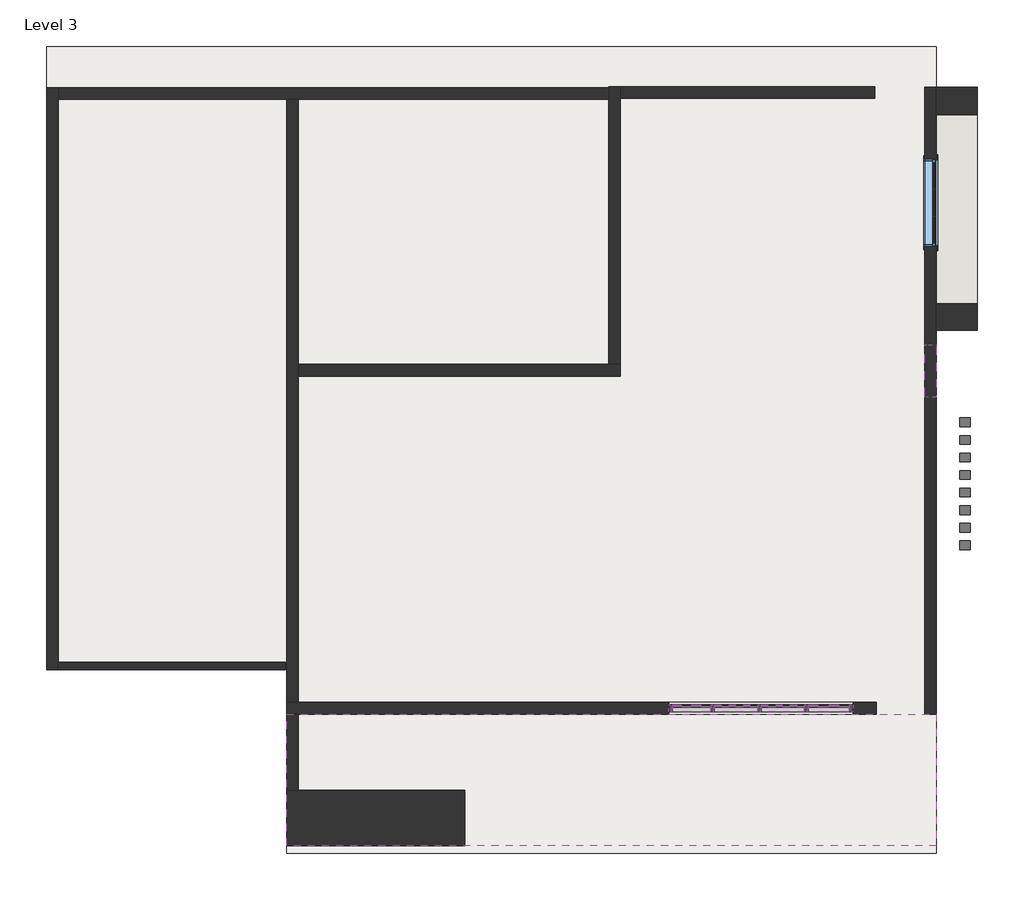
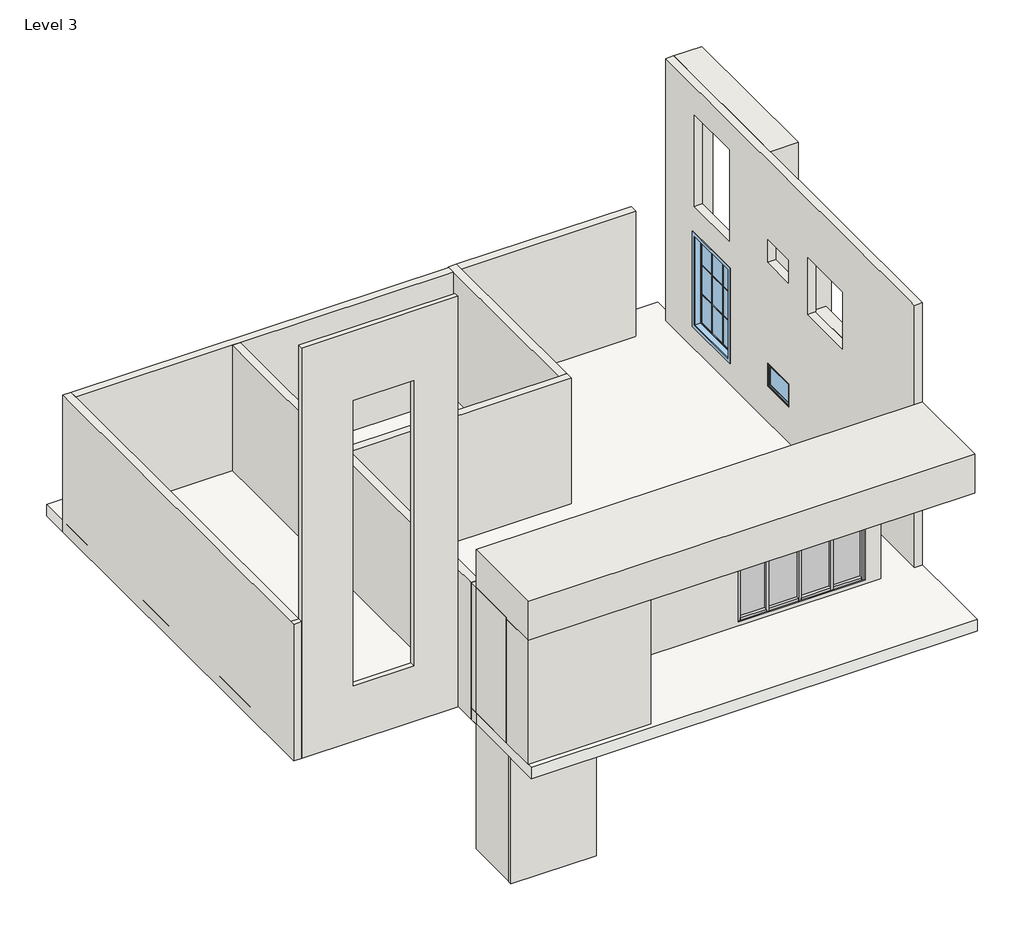
# One storey, incomplete: 22 members, 15 walls, 8 plates, 8 proxies, 2 windows, 1 roof.
"""IFC4 building model written with IfcOpenShell, lengths in millimetres."""

from ifc_helpers import new_model, si_unit, frame, origin, place, context, project, spatial, polyline, outline, extrude, faceted_brep, transform, mapped, element, save
from components import member_424e4c0f, member_61742b2b, member_5ade0aff, member_4d884067, member_c8ba4a72, member_20537117, member_aa870034, member_3a21dca5, member_2ee2964b, member_c33c434a, system_panel_glazed_10e47eeb, system_panel_glazed_d00a1739, system_panel_glazed_0ca22ccd, system_panel_glazed_ae16f783, system_panel_glazed_8c1b86c6, system_panel_glazed_afa25fb8, walls_1_walls_1_5166138d, walls_2_walls_2_a00b9660, walls_3_walls_3_551fdec1, window_41dcc157, window_57c3ee1c

model = new_model("IFC4")

# Units and contexts
model_context = context("Model", 3, world=origin())
ifc_project = project(units=[si_unit("LENGTHUNIT", "METRE", prefix="MILLI")], contexts=[model_context])

# Site, building, storey
site = spatial("IfcSite", under=ifc_project)
building = spatial("IfcBuilding", under=site)
storey = spatial("IfcBuildingStorey", under=building, Name="Level 3", Elevation=7315.2)

# Proxies
placement = place(None, origin())
element("IfcBuildingElementProxy", 1, Name="Reveal", ObjectType="Reveal", at=placement, inside=storey, context=model_context, shape_type="SweptSolid", body=[
    extrude(outline(polyline([(6653.2312442, 1993.3798743), (6470.3512442, 1993.3798743), (6470.3512442, 2145.7798743), (6653.2312442, 2145.7798743), (6653.2312442, 1993.3798743)])), frame((0.0, 0.0, 7620.0), z_axis=(0.0, 0.0, 1.0), x_axis=(1.0, 0.0, 0.0)), (0.0, 0.0, 1.0), 2067.2126797),
])
element("IfcBuildingElementProxy", 2, Name="Reveal", ObjectType="Reveal", at=placement, inside=storey, context=model_context, shape_type="SweptSolid", body=[
    extrude(outline(polyline([(6653.2312442, 2298.1798743), (6470.3512442, 2298.1798743), (6470.3512442, 2450.5798743), (6653.2312442, 2450.5798743), (6653.2312442, 2298.1798743)])), frame((0.0, 0.0, 7620.0), z_axis=(0.0, 0.0, 1.0), x_axis=(1.0, 0.0, 0.0)), (0.0, 0.0, 1.0), 2067.2126797),
])
element("IfcBuildingElementProxy", 3, Name="Reveal", ObjectType="Reveal", at=placement, inside=storey, context=model_context, shape_type="SweptSolid", body=[
    extrude(outline(polyline([(6653.2312442, 2602.9798743), (6470.3512442, 2602.9798743), (6470.3512442, 2755.3798743), (6653.2312442, 2755.3798743), (6653.2312442, 2602.9798743)])), frame((0.0, 0.0, 7620.0), z_axis=(0.0, 0.0, 1.0), x_axis=(1.0, 0.0, 0.0)), (0.0, 0.0, 1.0), 2067.2126797),
])
element("IfcBuildingElementProxy", 4, Name="Reveal", ObjectType="Reveal", at=placement, inside=storey, context=model_context, shape_type="SweptSolid", body=[
    extrude(outline(polyline([(6653.2312442, 2907.7798743), (6470.3512442, 2907.7798743), (6470.3512442, 3060.1798743), (6653.2312442, 3060.1798743), (6653.2312442, 2907.7798743)])), frame((0.0, 0.0, 7620.0), z_axis=(0.0, 0.0, 1.0), x_axis=(1.0, 0.0, 0.0)), (0.0, 0.0, 1.0), 2067.2126797),
])
element("IfcBuildingElementProxy", 5, Name="Reveal", ObjectType="Reveal", at=placement, inside=storey, context=model_context, shape_type="SweptSolid", body=[
    extrude(outline(polyline([(6653.2312442, 3212.5798743), (6470.3512442, 3212.5798743), (6470.3512442, 3364.9798743), (6653.2312442, 3364.9798743), (6653.2312442, 3212.5798743)])), frame((0.0, 0.0, 7620.0), z_axis=(0.0, 0.0, 1.0), x_axis=(1.0, 0.0, 0.0)), (0.0, 0.0, 1.0), 2067.2126797),
])
element("IfcBuildingElementProxy", 6, Name="Reveal", ObjectType="Reveal", at=placement, inside=storey, context=model_context, shape_type="SweptSolid", body=[
    extrude(outline(polyline([(6653.2312442, 3517.3798743), (6470.3512442, 3517.3798743), (6470.3512442, 3669.7798743), (6653.2312442, 3669.7798743), (6653.2312442, 3517.3798743)])), frame((0.0, 0.0, 7620.0), z_axis=(0.0, 0.0, 1.0), x_axis=(1.0, 0.0, 0.0)), (0.0, 0.0, 1.0), 2067.2126797),
])
element("IfcBuildingElementProxy", 7, Name="Reveal", ObjectType="Reveal", at=placement, inside=storey, context=model_context, shape_type="SweptSolid", body=[
    extrude(outline(polyline([(6653.2312442, 3822.1798743), (6470.3512442, 3822.1798743), (6470.3512442, 3974.5798743), (6653.2312442, 3974.5798743), (6653.2312442, 3822.1798743)])), frame((0.0, 0.0, 7620.0), z_axis=(0.0, 0.0, 1.0), x_axis=(1.0, 0.0, 0.0)), (0.0, 0.0, 1.0), 2067.2126797),
])
element("IfcBuildingElementProxy", 8, Name="Reveal", ObjectType="Reveal", at=placement, inside=storey, context=model_context, shape_type="SweptSolid", body=[
    extrude(outline(polyline([(6653.2312442, 4126.9798743), (6470.3512442, 4126.9798743), (6470.3512442, 4279.3798743), (6653.2312442, 4279.3798743), (6653.2312442, 4126.9798743)])), frame((0.0, 0.0, 7620.0), z_axis=(0.0, 0.0, 1.0), x_axis=(1.0, 0.0, 0.0)), (0.0, 0.0, 1.0), 2067.2126797),
])

# Members
member_shape = member_424e4c0f(model_context)
element("IfcMember", 9, ObjectType="Rectangular Mullion : 2.5\" x 5\" rectangular", at=placement, inside=storey, context=model_context, shape_type="MappedRepresentation", body=[
    mapped(member_shape, transform((3771.7551378, -759.3451257, 9949.3840877), x_axis=(0.0, 0.0, 1.0), y_axis=(0.0, -1.0, 0.0), z_axis=(1.0, 0.0, 0.0))),
])
element("IfcMember", 10, ObjectType="Rectangular Mullion : 2.5\" x 5\" rectangular", at=placement, inside=storey, context=model_context, shape_type="MappedRepresentation", body=[
    mapped(member_shape, transform((2958.9382617, -759.3451257, 9949.3840877), x_axis=(0.0, 0.0, 1.0), y_axis=(0.0, -1.0, 0.0), z_axis=(1.0, 0.0, 0.0))),
])
member_2_shape = member_61742b2b(model_context)
element("IfcMember", 11, ObjectType="Rectangular Mullion : 2.5\" x 5\" rectangular", at=placement, inside=storey, context=model_context, shape_type="MappedRepresentation", body=[
    mapped(member_2_shape, transform((2177.8713856, -759.3451257, 9949.3840877), x_axis=(1.0, 0.0, 0.0), y_axis=(0.0, -1.0, 0.0), z_axis=(0.0, 0.0, -1.0))),
])
element("IfcMember", 12, ObjectType="Rectangular Mullion : 2.5\" x 5\" rectangular", at=placement, inside=storey, context=model_context, shape_type="MappedRepresentation", body=[
    mapped(member_2_shape, transform((2990.6882617, -759.3451257, 9949.3840877), x_axis=(1.0, 0.0, 0.0), y_axis=(0.0, -1.0, 0.0), z_axis=(0.0, 0.0, -1.0))),
])
element("IfcMember", 13, ObjectType="Rectangular Mullion : 2.5\" x 5\" rectangular", at=placement, inside=storey, context=model_context, shape_type="MappedRepresentation", body=[
    mapped(member_2_shape, transform((3803.5051378, -759.3451257, 9949.3840877), x_axis=(1.0, 0.0, 0.0), y_axis=(0.0, -1.0, 0.0), z_axis=(0.0, 0.0, -1.0))),
])
member_3_shape = member_5ade0aff(model_context)
element("IfcMember", 14, ObjectType="Rectangular Mullion : 2.5\" x 5\" rectangular", at=placement, inside=storey, context=model_context, shape_type="MappedRepresentation", body=[
    mapped(member_3_shape, transform((3771.7551378, -759.3451257, 10711.3840877), x_axis=(0.0, 0.0, 1.0), y_axis=(0.0, -1.0, 0.0), z_axis=(1.0, 0.0, 0.0))),
])
element("IfcMember", 15, ObjectType="Rectangular Mullion : 2.5\" x 5\" rectangular", at=placement, inside=storey, context=model_context, shape_type="MappedRepresentation", body=[
    mapped(member_3_shape, transform((2958.9382617, -759.3451257, 10711.3840877), x_axis=(0.0, 0.0, 1.0), y_axis=(0.0, -1.0, 0.0), z_axis=(1.0, 0.0, 0.0))),
])
member_4_shape = member_4d884067(model_context)
element("IfcMember", 16, ObjectType="Rectangular Mullion : 2.5\" x 5\" rectangular", at=placement, inside=storey, context=model_context, shape_type="MappedRepresentation", body=[
    mapped(member_4_shape, transform((2177.8713856, -759.3451257, 7721.6), x_axis=(1.0, 0.0, 0.0), y_axis=(0.0, -1.0, 0.0), z_axis=(0.0, 0.0, -1.0))),
])
element("IfcMember", 17, ObjectType="Rectangular Mullion : 2.5\" x 5\" rectangular", at=placement, inside=storey, context=model_context, shape_type="MappedRepresentation", body=[
    mapped(member_4_shape, transform((2990.6882617, -759.3451257, 7721.6), x_axis=(1.0, 0.0, 0.0), y_axis=(0.0, -1.0, 0.0), z_axis=(0.0, 0.0, -1.0))),
])
element("IfcMember", 18, ObjectType="Rectangular Mullion : 2.5\" x 5\" rectangular", at=placement, inside=storey, context=model_context, shape_type="MappedRepresentation", body=[
    mapped(member_4_shape, transform((3803.5051378, -759.3451257, 7721.6), x_axis=(1.0, 0.0, 0.0), y_axis=(0.0, -1.0, 0.0), z_axis=(0.0, 0.0, -1.0))),
])
element("IfcMember", 19, ObjectType="Rectangular Mullion : 2.5\" x 5\" rectangular", at=placement, inside=storey, context=model_context, shape_type="MappedRepresentation", body=[
    mapped(member_3_shape, transform((3022.4382617, -759.3451257, 7721.6), x_axis=(0.0, 0.0, -1.0), y_axis=(0.0, -1.0, 0.0), z_axis=(-1.0, 0.0, 0.0))),
])
element("IfcMember", 20, ObjectType="Rectangular Mullion : 2.5\" x 5\" rectangular", at=placement, inside=storey, context=model_context, shape_type="MappedRepresentation", body=[
    mapped(member_3_shape, transform((2209.6213856, -759.3451257, 7721.6), x_axis=(0.0, 0.0, -1.0), y_axis=(0.0, -1.0, 0.0), z_axis=(-1.0, 0.0, 0.0))),
])
member_5_shape = member_c8ba4a72(model_context)
element("IfcMember", 21, ObjectType="Rectangular Mullion : 2.5\" x 5\" rectangular", at=placement, inside=storey, context=model_context, shape_type="MappedRepresentation", body=[
    mapped(member_5_shape, transform((4552.8220139, -759.3451257, 9949.3840877), x_axis=(0.0, 0.0, 1.0), y_axis=(0.0, -1.0, 0.0), z_axis=(1.0, 0.0, 0.0))),
])
member_6_shape = member_20537117(model_context)
element("IfcMember", 22, ObjectType="Rectangular Mullion : 2.5\" x 5\" rectangular", at=placement, inside=storey, context=model_context, shape_type="MappedRepresentation", body=[
    mapped(member_6_shape, transform((4552.8220139, -759.3451257, 10711.3840877), x_axis=(0.0, 0.0, 1.0), y_axis=(0.0, -1.0, 0.0), z_axis=(1.0, 0.0, 0.0))),
])
element("IfcMember", 23, ObjectType="Rectangular Mullion : 2.5\" x 5\" rectangular", at=placement, inside=storey, context=model_context, shape_type="MappedRepresentation", body=[
    mapped(member_6_shape, transform((3835.2551378, -759.3451257, 7721.6), x_axis=(0.0, 0.0, -1.0), y_axis=(0.0, -1.0, 0.0), z_axis=(-1.0, 0.0, 0.0))),
])
member_7_shape = member_aa870034(model_context)
element("IfcMember", 24, ObjectType="Rectangular Mullion : 2.5\" x 5\" rectangular", at=placement, inside=storey, context=model_context, shape_type="MappedRepresentation", body=[
    mapped(member_7_shape, transform((4616.3220139, -759.3451257, 9949.3840877), x_axis=(1.0, 0.0, 0.0), y_axis=(0.0, -1.0, 0.0), z_axis=(0.0, 0.0, -1.0))),
])
member_8_shape = member_3a21dca5(model_context)
element("IfcMember", 25, ObjectType="Rectangular Mullion : 2.5\" x 5\" rectangular", at=placement, inside=storey, context=model_context, shape_type="MappedRepresentation", body=[
    mapped(member_8_shape, transform((4616.3220139, -759.3451257, 7721.6), x_axis=(1.0, 0.0, 0.0), y_axis=(0.0, -1.0, 0.0), z_axis=(0.0, 0.0, -1.0))),
])
member_9_shape = member_2ee2964b(model_context)
element("IfcMember", 26, ObjectType="Rectangular Mullion : 2.5\" x 5\" rectangular", at=placement, inside=storey, context=model_context, shape_type="MappedRepresentation", body=[
    mapped(member_9_shape, transform((2146.1213856, -759.3451257, 9949.3840877), x_axis=(0.0, 0.0, 1.0), y_axis=(0.0, -1.0, 0.0), z_axis=(1.0, 0.0, 0.0))),
])
member_10_shape = member_c33c434a(model_context)
element("IfcMember", 27, ObjectType="Rectangular Mullion : 2.5\" x 5\" rectangular", at=placement, inside=storey, context=model_context, shape_type="MappedRepresentation", body=[
    mapped(member_10_shape, transform((2146.1213856, -759.3451257, 10711.3840877), x_axis=(0.0, 0.0, 1.0), y_axis=(0.0, -1.0, 0.0), z_axis=(1.0, 0.0, 0.0))),
])
element("IfcMember", 28, ObjectType="Rectangular Mullion : 2.5\" x 5\" rectangular", at=placement, inside=storey, context=model_context, shape_type="MappedRepresentation", body=[
    mapped(member_10_shape, transform((1479.3713856, -759.3451257, 7721.6), x_axis=(0.0, 0.0, -1.0), y_axis=(0.0, -1.0, 0.0), z_axis=(-1.0, 0.0, 0.0))),
])
element("IfcMember", 29, ObjectType="Rectangular Mullion : 2.5\" x 5\" rectangular", at=placement, inside=storey, context=model_context, shape_type="MappedRepresentation", body=[
    mapped(member_8_shape, transform((1415.8713856, -759.3451257, 9949.3840877), x_axis=(-1.0, 0.0, 0.0), y_axis=(0.0, -1.0, 0.0), z_axis=(0.0, 0.0, 1.0))),
])
element("IfcMember", 30, ObjectType="Rectangular Mullion : 2.5\" x 5\" rectangular", at=placement, inside=storey, context=model_context, shape_type="MappedRepresentation", body=[
    mapped(member_7_shape, transform((1415.8713856, -759.3451257, 10711.3840877), x_axis=(-1.0, 0.0, 0.0), y_axis=(0.0, -1.0, 0.0), z_axis=(0.0, 0.0, 1.0))),
])

# Plates
system_panel_glazed_shape = system_panel_glazed_10e47eeb(model_context)
element("IfcPlate", 31, ObjectType="System Panel : Glazed", at=placement, inside=storey, context=model_context, shape_type="MappedRepresentation", body=[
    mapped(system_panel_glazed_shape, transform((2584.2798237, -759.3451257, 9981.1340877), x_axis=(1.0, 0.0, 0.0), y_axis=(0.0, 1.0, 0.0), z_axis=(0.0, 0.0, 1.0))),
])
element("IfcPlate", 32, ObjectType="System Panel : Glazed", at=placement, inside=storey, context=model_context, shape_type="MappedRepresentation", body=[
    mapped(system_panel_glazed_shape, transform((3397.0966998, -759.3451257, 9981.1340877), x_axis=(1.0, 0.0, 0.0), y_axis=(0.0, 1.0, 0.0), z_axis=(0.0, 0.0, 1.0))),
])
system_panel_glazed_2_shape = system_panel_glazed_d00a1739(model_context)
element("IfcPlate", 33, ObjectType="System Panel : Glazed", at=placement, inside=storey, context=model_context, shape_type="MappedRepresentation", body=[
    mapped(system_panel_glazed_2_shape, transform((2584.2798237, -759.3451257, 7785.1), x_axis=(1.0, 0.0, 0.0), y_axis=(0.0, 1.0, 0.0), z_axis=(0.0, 0.0, 1.0))),
])
element("IfcPlate", 34, ObjectType="System Panel : Glazed", at=placement, inside=storey, context=model_context, shape_type="MappedRepresentation", body=[
    mapped(system_panel_glazed_2_shape, transform((3397.0966998, -759.3451257, 7785.1), x_axis=(1.0, 0.0, 0.0), y_axis=(0.0, 1.0, 0.0), z_axis=(0.0, 0.0, 1.0))),
])
system_panel_glazed_3_shape = system_panel_glazed_0ca22ccd(model_context)
element("IfcPlate", 35, ObjectType="System Panel : Glazed", at=placement, inside=storey, context=model_context, shape_type="MappedRepresentation", body=[
    mapped(system_panel_glazed_3_shape, transform((4194.0385758, -759.3451257, 7785.1), x_axis=(1.0, 0.0, 0.0), y_axis=(0.0, 1.0, 0.0), z_axis=(0.0, 0.0, 1.0))),
])
system_panel_glazed_4_shape = system_panel_glazed_ae16f783(model_context)
element("IfcPlate", 36, ObjectType="System Panel : Glazed", at=placement, inside=storey, context=model_context, shape_type="MappedRepresentation", body=[
    mapped(system_panel_glazed_4_shape, transform((4194.0385758, -759.3451257, 9981.1340877), x_axis=(1.0, 0.0, 0.0), y_axis=(0.0, 1.0, 0.0), z_axis=(0.0, 0.0, 1.0))),
])
system_panel_glazed_5_shape = system_panel_glazed_8c1b86c6(model_context)
element("IfcPlate", 37, ObjectType="System Panel : Glazed", at=placement, inside=storey, context=model_context, shape_type="MappedRepresentation", body=[
    mapped(system_panel_glazed_5_shape, transform((1812.7463856, -759.3451257, 7785.1), x_axis=(1.0, 0.0, 0.0), y_axis=(0.0, 1.0, 0.0), z_axis=(0.0, 0.0, 1.0))),
])
system_panel_glazed_6_shape = system_panel_glazed_afa25fb8(model_context)
element("IfcPlate", 38, ObjectType="System Panel : Glazed", at=placement, inside=storey, context=model_context, shape_type="MappedRepresentation", body=[
    mapped(system_panel_glazed_6_shape, transform((1812.7463856, -759.3451257, 9981.1340877), x_axis=(1.0, 0.0, 0.0), y_axis=(0.0, 1.0, 0.0), z_axis=(0.0, 0.0, 1.0))),
])

# Roof
element("IfcRoof", 39, ObjectType="Generic - 12\"", at=placement, inside=storey, context=model_context, shape_type="SweptSolid", body=[
    extrude(outline(polyline([(-9379.3749149, 10724.4481987), (6063.8250851, 10724.4481987), (6063.8250851, -3270.9518013), (-5213.7749149, -3270.9518013), (-5213.7749149, 2.6548743), (-9379.3749149, 2.6548743), (-9379.3749149, 10724.4481987)])), frame((0.0, 0.0, 7315.2), z_axis=(0.0, 0.0, 1.0), x_axis=(1.0, 0.0, 0.0)), (0.0, 0.0, 1.0), 304.8),
])

# Walls
element("IfcWall", 40, ObjectType="Generic - 4\" Brick", at=placement, inside=storey, context=model_context, shape_type="Brep", body=[
    faceted_brep([(-5213.7749149, -2381.9518013, 3962.4), (-3054.7749149, -2381.9518013, 3962.4), (-3054.7749149, -2381.9518013, 7315.2), (-5213.7749149, -2381.9518013, 7315.2), (-5213.7749149, -2280.3518013, 3962.4), (-5213.7749149, -2280.3518013, 3979.4508154), (-5213.7749149, -2280.3518013, 7315.2), (-5086.7749149, -2280.3518013, 7315.2), (-3054.7749149, -2280.3518013, 7315.2), (-3054.7749149, -2280.3518013, 3962.4)], [[[0, 1, 2, 3]], [[4, 5, 6, 7, 8, 9]], [[1, 0, 4, 9]], [[2, 1, 9, 8]], [[3, 2, 8, 7, 6]], [[0, 3, 6, 5, 4]]]),
])
element("IfcWall", 41, ObjectType="Generic - 5\"", at=placement, inside=storey, context=model_context, shape_type="Brep", body=[
    faceted_brep([(-9176.1749149, -86.2451257, 7315.2), (-5232.8249149, -86.2451257, 7315.2), (-5232.8249149, -86.2451257, 18288.0), (-9176.1749149, -86.2451257, 18288.0), (-9176.1749149, -86.2451257, 14630.4), (-9176.1749149, -86.2451257, 10972.8), (-7864.8999149, -86.2451257, 8799.9445366), (-7864.8999149, -86.2451257, 16419.9445366), (-6340.8999149, -86.2451257, 16419.9445366), (-6340.8999149, -86.2451257, 8799.9445366), (-5232.8249149, 40.7548743, 7315.2), (-9176.1749149, 40.7548743, 7315.2), (-9176.1749149, 40.7548743, 18288.0), (-5232.8249149, 40.7548743, 18288.0), (-7864.8999149, 40.7548743, 16419.9445366), (-7864.8999149, 40.7548743, 8799.9445366), (-6340.8999149, 40.7548743, 8799.9445366), (-6340.8999149, 40.7548743, 16419.9445366)], [[[0, 1, 2, 3, 4, 5], [6, 7, 8, 9]], [[10, 11, 12, 13], [14, 15, 16, 17]], [[1, 0, 11, 10]], [[2, 1, 10, 13]], [[3, 2, 13, 12]], [[3, 12, 11, 0, 5, 4]], [[14, 7, 6, 15]], [[15, 6, 9, 16]], [[16, 9, 8, 17]], [[7, 14, 17, 8]]]),
])
element("IfcWall", 42, ObjectType="Generic - 5\"", at=placement, inside=storey, context=model_context, shape_type="SweptSolid", body=[
    extrude(outline(polyline([(-5213.7749149, -2280.3518013), (-5213.7749149, -860.9451257), (-5086.7749149, -860.9451257), (-5086.7749149, -2280.3518013), (-5213.7749149, -2280.3518013)])), frame((0.0, 0.0, 3979.4508154), z_axis=(0.0, 0.0, 1.0), x_axis=(1.0, 0.0, 0.0)), (0.0, 0.0, 1.0), 3335.7491846),
])
element("IfcWall", 43, ObjectType="Generic - 8\"", at=placement, inside=storey, context=model_context, shape_type="Brep", body=[
    faceted_brep([(-5213.7749149, -657.7451257, 7315.2), (-5213.7749149, -657.7451257, 10972.8), (-5010.5749149, -657.7451257, 10972.8), (4997.0250851, -657.7451257, 10972.8), (5016.0750851, -657.7451257, 10972.8), (5016.0750851, -657.7451257, 7620.0), (5016.0750851, -657.7451257, 7315.2), (-5010.5749149, -657.7451257, 7315.2), (4616.3220139, -657.7451257, 10711.3840877), (1415.8713856, -657.7451257, 10711.3840877), (1415.8713856, -657.7451257, 7721.6), (4616.3220139, -657.7451257, 7721.6), (-5213.7749149, -860.9451257, 10972.8), (-5213.7749149, -860.9451257, 7620.0), (-5213.7749149, -860.9451257, 7315.2), (5016.0750851, -860.9451257, 7315.2), (5016.0750851, -860.9451257, 7620.0), (5016.0750851, -860.9451257, 10972.8), (4997.0250851, -860.9451257, 10972.8), (-5010.5749149, -860.9451257, 10972.8), (4616.3220139, -860.9451257, 10711.3840877), (4616.3220139, -860.9451257, 7721.6), (1415.8713856, -860.9451257, 7721.6), (1415.8713856, -860.9451257, 10711.3840877)], [[[0, 1, 2, 3, 4, 5, 6, 7], [8, 9, 10, 11]], [[12, 13, 14, 15, 16, 17, 18, 19], [20, 21, 22, 23]], [[0, 7, 6, 15, 14]], [[6, 5, 4, 17, 16, 15]], [[4, 3, 18, 17]], [[3, 2, 1, 12, 19, 18]], [[0, 14, 13, 12, 1]], [[9, 8, 20, 23]], [[10, 9, 23, 22]], [[11, 10, 22, 21]], [[8, 11, 21, 20]]]),
])
element("IfcWall", 44, ObjectType="Generic - 8\"", at=placement, inside=storey, context=model_context, shape_type="Brep", body=[
    faceted_brep([(-5010.5749149, -657.7451257, 10972.8), (-5010.5749149, -657.7451257, 7315.2), (-5010.5749149, 5006.4548743, 7315.2), (-5010.5749149, 5209.6548743, 7315.2), (-5010.5749149, 9807.0548743, 7315.2), (-5010.5749149, 9807.0548743, 10972.8), (-5010.5749149, 5209.6548743, 10972.8), (-5010.5749149, 5006.4548743, 10972.8), (-5213.7749149, -657.7451257, 7315.2), (-5213.7749149, -657.7451257, 10972.8), (-5213.7749149, 40.7548743, 10972.8), (-5213.7749149, 9807.0548743, 10972.8), (-5213.7749149, 9807.0548743, 7315.2)], [[[0, 1, 2, 3, 4, 5, 6, 7]], [[8, 9, 10, 11, 12]], [[4, 3, 2, 1, 8, 12]], [[5, 4, 12, 11]], [[0, 7, 6, 5, 11, 10, 9]], [[0, 9, 8, 1]]]),
])
element("IfcWall", 45, ObjectType="Generic - 8\"", at=placement, inside=storey, context=model_context, shape_type="Brep", body=[
    faceted_brep([(-5010.5749149, 5006.4548743, 7315.2), (577.4250851, 5006.4548743, 7315.2), (577.4250851, 5006.4548743, 10972.8), (-5010.5749149, 5006.4548743, 10972.8), (-5010.5749149, 5209.6548743, 7315.2), (-5010.5749149, 5209.6548743, 10972.8), (374.2250851, 5209.6548743, 10972.8), (577.4250851, 5209.6548743, 10972.8), (577.4250851, 5209.6548743, 7315.2), (374.2250851, 5209.6548743, 7315.2)], [[[0, 1, 2, 3]], [[4, 5, 6, 7, 8, 9]], [[1, 0, 4, 9, 8]], [[0, 3, 5, 4]], [[2, 1, 8, 7]], [[3, 2, 7, 6, 5]]]),
])
element("IfcWall", 46, ObjectType="Generic - 8\"", at=placement, inside=storey, context=model_context, shape_type="Brep", body=[
    faceted_brep([(577.4250851, 5209.6548743, 7315.2), (577.4250851, 9826.1048743, 7315.2), (577.4250851, 10029.3048743, 7315.2), (577.4250851, 10029.3048743, 10972.8), (577.4250851, 9826.1048743, 10972.8), (577.4250851, 5209.6548743, 10972.8), (374.2250851, 5209.6548743, 7315.2), (374.2250851, 5209.6548743, 10972.8), (374.2250851, 9807.0548743, 10972.8), (374.2250851, 10010.2548743, 10972.8), (374.2250851, 10029.3048743, 10972.8), (374.2250851, 10029.3048743, 7315.2), (374.2250851, 10010.2548743, 7315.2), (374.2250851, 9807.0548743, 7315.2)], [[[0, 1, 2, 3, 4, 5]], [[6, 7, 8, 9, 10, 11, 12, 13]], [[2, 1, 0, 6, 13, 12, 11]], [[0, 5, 7, 6]], [[3, 2, 11, 10]], [[5, 4, 3, 10, 9, 8, 7]]]),
])
element("IfcWall", 47, ObjectType="Generic - 8\"", at=placement, inside=storey, context=model_context, shape_type="SweptSolid", body=[
    extrude(outline(polyline([(4997.0250851, 9826.1048743), (577.4250851, 9826.1048743), (577.4250851, 10029.3048743), (4997.0250851, 10029.3048743), (4997.0250851, 9826.1048743)])), frame((0.0, 0.0, 7315.2), z_axis=(0.0, 0.0, 1.0), x_axis=(1.0, 0.0, 0.0)), (0.0, 0.0, 1.0), 3657.6),
])
element("IfcWall", 48, ObjectType="Generic - 8\"", at=placement, inside=storey, context=model_context, shape_type="Brep", body=[
    faceted_brep([(5860.6250851, 10019.7798743, 7315.2), (5860.6250851, -860.9451257, 7315.2), (5860.6250851, -860.9451257, 7620.0), (5860.6250851, -860.9451257, 14630.4), (5860.6250851, -657.7451257, 14630.4), (5860.6250851, 9816.5798743, 14630.4), (5860.6250851, 10019.7798743, 14630.4), (5860.6250851, 10019.7798743, 7620.0), (5860.6250851, 2288.6548743, 13078.2899453), (5860.6250851, 2288.6548743, 11554.2899453), (5860.6250851, 3812.6548743, 11554.2899453), (5860.6250851, 3812.6548743, 13078.2899453), (5860.6250851, 7251.1798743, 13868.4), (5860.6250851, 7251.1798743, 11430.0), (5860.6250851, 8775.1798743, 11430.0), (5860.6250851, 8775.1798743, 13868.4), (5860.6250851, 7251.1798743, 10687.6524407), (5860.6250851, 7251.1798743, 8249.2524407), (5860.6250851, 8775.1798743, 8249.2524407), (5860.6250851, 8775.1798743, 10687.6524407), (5860.6250851, 5565.2548743, 12496.8), (5860.6250851, 4650.8548743, 12496.8), (5860.6250851, 4650.8548743, 11887.2), (5860.6250851, 5565.2548743, 11887.2), (5860.6250851, 5549.3798743, 9195.1883617), (5860.6250851, 4634.9798743, 9195.1883617), (5860.6250851, 4634.9798743, 8585.5883617), (5860.6250851, 5549.3798743, 8585.5883617), (6063.8250851, 10019.7798743, 7315.2), (6063.8250851, 10019.7798743, 14630.4), (6063.8250851, -860.9451257, 14630.4), (6063.8250851, -860.9451257, 7315.2), (6063.8250851, 2288.6548743, 13078.2899453), (6063.8250851, 3812.6548743, 13078.2899453), (6063.8250851, 3812.6548743, 11554.2899453), (6063.8250851, 2288.6548743, 11554.2899453), (6063.8250851, 7251.1798743, 13868.4), (6063.8250851, 8775.1798743, 13868.4), (6063.8250851, 8775.1798743, 11430.0), (6063.8250851, 7251.1798743, 11430.0), (6063.8250851, 7251.1798743, 10687.6524407), (6063.8250851, 8775.1798743, 10687.6524407), (6063.8250851, 8775.1798743, 8249.2524407), (6063.8250851, 7251.1798743, 8249.2524407), (6063.8250851, 5565.2548743, 12496.8), (6063.8250851, 5565.2548743, 11887.2), (6063.8250851, 4650.8548743, 11887.2), (6063.8250851, 4650.8548743, 12496.8), (6063.8250851, 5549.3798743, 9195.1883617), (6063.8250851, 5549.3798743, 8585.5883617), (6063.8250851, 4634.9798743, 8585.5883617), (6063.8250851, 4634.9798743, 9195.1883617)], [[[0, 1, 2, 3, 4, 5, 6, 7], [8, 9, 10, 11], [12, 13, 14, 15], [16, 17, 18, 19], [20, 21, 22, 23], [24, 25, 26, 27]], [[28, 29, 30, 31], [32, 33, 34, 35], [36, 37, 38, 39], [40, 41, 42, 43], [44, 45, 46, 47], [48, 49, 50, 51]], [[1, 0, 28, 31]], [[0, 7, 6, 29, 28]], [[3, 2, 1, 31, 30]], [[9, 8, 32, 35]], [[10, 9, 35, 34]], [[11, 10, 34, 33]], [[8, 11, 33, 32]], [[13, 12, 36, 39]], [[14, 13, 39, 38]], [[15, 14, 38, 37]], [[12, 15, 37, 36]], [[17, 16, 40, 43]], [[18, 17, 43, 42]], [[19, 18, 42, 41]], [[16, 19, 41, 40]], [[45, 44, 20, 23]], [[46, 45, 23, 22]], [[47, 46, 22, 21]], [[44, 47, 21, 20]], [[49, 48, 24, 27]], [[50, 49, 27, 26]], [[51, 50, 26, 25]], [[48, 51, 25, 24]], [[6, 5, 4, 3, 30, 29]]]),
])
element("IfcWall", 49, ObjectType="Generic - 8\"", at=placement, inside=storey, context=model_context, shape_type="Brep", body=[
    faceted_brep([(-9176.1749149, -86.2451257, 7315.2), (-9176.1749149, 40.7548743, 7315.2), (-9176.1749149, 9807.0548743, 7315.2), (-9176.1749149, 10010.2548743, 7315.2), (-9176.1749149, 10010.2548743, 10972.8), (-9176.1749149, 9807.0548743, 10972.8), (-9176.1749149, 40.7548743, 10972.8), (-9176.1749149, -86.2451257, 10972.8), (-9379.3749149, -86.2451257, 7315.2), (-9379.3749149, -86.2451257, 10972.8), (-9379.3749149, 40.7548743, 10972.8), (-9379.3749149, 10010.2548743, 10972.8), (-9379.3749149, 10010.2548743, 7315.2)], [[[0, 1, 2, 3, 4, 5, 6, 7]], [[8, 9, 10, 11, 12]], [[3, 2, 1, 0, 8, 12]], [[4, 3, 12, 11]], [[7, 6, 10, 9]], [[6, 5, 4, 11, 10]], [[0, 7, 9, 8]]]),
])
element("IfcWall", 50, ObjectType="Generic - 8\"", at=placement, inside=storey, context=model_context, shape_type="Brep", body=[
    faceted_brep([(-9176.1749149, 9807.0548743, 7315.2), (-5213.7749149, 9807.0548743, 7315.2), (-5010.5749149, 9807.0548743, 7315.2), (374.2250851, 9807.0548743, 7315.2), (374.2250851, 9807.0548743, 10972.8), (-5010.5749149, 9807.0548743, 10972.8), (-5213.7749149, 9807.0548743, 10972.8), (-9176.1749149, 9807.0548743, 10972.8), (-9176.1749149, 10010.2548743, 7315.2), (-9176.1749149, 10010.2548743, 10972.8), (374.2250851, 10010.2548743, 10972.8), (374.2250851, 10010.2548743, 7315.2)], [[[0, 1, 2, 3, 4, 5, 6, 7]], [[8, 9, 10, 11]], [[3, 2, 1, 0, 8, 11]], [[4, 3, 11, 10]], [[0, 7, 9, 8]], [[7, 6, 5, 4, 10, 9]]]),
])
element("IfcWall", 51, ObjectType="Generic - 8\"", at=placement, inside=storey, context=model_context, shape_type="SweptSolid", body=[
    extrude(outline(polyline([(-5213.7749149, -2181.7451257), (-5213.7749149, -860.9451257), (-5010.5749149, -860.9451257), (-5010.5749149, -2181.7451257), (-5213.7749149, -2181.7451257)])), frame((0.0, 0.0, 7620.0), z_axis=(0.0, 0.0, 1.0), x_axis=(1.0, 0.0, 0.0)), (0.0, 0.0, 1.0), 3352.8),
])
walls_1_walls_1_shape = walls_1_walls_1_5166138d(model_context)
element("IfcWall", 52, ObjectType="Walls 1 : Walls 1", at=placement, inside=storey, context=model_context, shape_type="MappedRepresentation", body=[
    mapped(walls_1_walls_1_shape, transform((0.0, 0.0, 0.0), x_axis=(1.0, 0.0, 0.0), y_axis=(0.0, 1.0, 0.0), z_axis=(0.0, 0.0, 1.0))),
])
walls_2_walls_2_shape = walls_2_walls_2_a00b9660(model_context)
element("IfcWall", 53, ObjectType="Walls 2 : Walls 2", at=placement, inside=storey, context=model_context, shape_type="MappedRepresentation", body=[
    mapped(walls_2_walls_2_shape, transform((0.0, 0.0, 0.0), x_axis=(1.0, 0.0, 0.0), y_axis=(0.0, 1.0, 0.0), z_axis=(0.0, 0.0, 1.0))),
])
walls_3_walls_3_shape = walls_3_walls_3_551fdec1(model_context)
element("IfcWall", 54, ObjectType="Walls 3 : Walls 3", at=placement, inside=storey, context=model_context, shape_type="MappedRepresentation", body=[
    mapped(walls_3_walls_3_shape, transform((0.0, 0.0, 0.0), x_axis=(1.0, 0.0, 0.0), y_axis=(0.0, 1.0, 0.0), z_axis=(0.0, 0.0, 1.0))),
])

# Windows
window_shape = window_41dcc157(model_context)
element("IfcWindow", 55, ObjectType="Casement 3x3 with Trim : 60\" x 96\"", at=placement, inside=storey, context=model_context, shape_type="MappedRepresentation", body=[
    mapped(window_shape, transform((5962.2250851, 8013.1798743, 7944.4524407), x_axis=(0.0, -1.0, 0.0), y_axis=(1.0, 0.0, 0.0), z_axis=(0.0, 0.0, 1.0))),
])
window_2_shape = window_57c3ee1c(model_context)
element("IfcWindow", 56, ObjectType="Fixed : 36\" x 24\"", at=placement, inside=storey, context=model_context, shape_type="MappedRepresentation", body=[
    mapped(window_2_shape, transform((5962.2250851, 5130.2798743, 7671.1883617), x_axis=(0.0, 1.0, 0.0), y_axis=(-1.0, 0.0, 0.0), z_axis=(0.0, 0.0, 1.0))),
])

save(model, "model.ifc")

# Revit data of these elements
# Type "Rectangular Mullion : 2.5\" x 5\" rectangular"
#   built-in parameter 1007304 = 0.416667 (stored number, unit not read)
#   built-in parameter 1007301 = 0.104167 (stored number, unit not read)
#   built-in parameter 1007300 = 0.104167 (stored number, unit not read)
# Type "System Panel : Glazed"
#   Construction Type Id = "GSP4R"
#   Analytic Construction = "1/8 in Pilkington single glazing"
#   Visual Light Transmittance = 0.9
#   Solar Heat Gain Coefficient = 0.86
#   Heat Transfer Coefficient (U) = 1.18115 BTU/(h·ft²·°F)
# Type "Generic - 12\""
#   Assembly Code = "B1020"
#   Layers, outside or top first: 1' - 0" no material (function 1)
# Type "Generic - 4\" Brick"
#   Assembly Code = "B2010"
#   Layers, outside or top first: 0' - 4" "Brick, Common" (function 1)
# Type "Generic - 5\""
#   Assembly Code = "B2010"
#   Layers, outside or top first: 0' - 5" no material (function 1)
# Type "Generic - 8\""
#   Assembly Code = "B2010"
#   Layers, outside or top first: 0' - 8" no material (function 1)
# Type "Casement 3x3 with Trim : 60\" x 96\""
#   Type Mark = "15"
#   Construction Type Id = "GSP4R"
#   Assembly Code = "B2020100"
#   Analytic Construction = "1/8 in Pilkington single glazing"
#   Visual Light Transmittance = 0.9
#   Solar Heat Gain Coefficient = 0.78
#   Heat Transfer Coefficient (U) = 0.6496 BTU/(h·ft²·°F)
#   Height = 8' - 0"
#   Default Sill Height = 1' - 0"
#   Trim Projection - Ext. = 0' - 0 1/2"
#   Trim Projection - Int. = 0' - 0 3/4"
#   Trim Width - Exterior = 0' - 3 1/2"
#   Trim Width - Interior = 0' - 3 1/2"
#   Width = 5' - 0"
#   Window Inset = 0' - 0 3/4"
#   Define Thermal Properties by = 1
#   Glass Pane Material = Glass
#   Sash Material = Sash
#   Trim Exterior Material = Trim
#   Trim Interior Material = Trim
#   Wall Closure = (empty or 0)
# Type "Fixed : 36\" x 24\""
#   Type Mark = "8"
#   Construction Type Id = "GSP4R"
#   Assembly Code = "B2020100"
#   Analytic Construction = "1/8 in Pilkington single glazing"
#   Visual Light Transmittance = 0.9
#   Solar Heat Gain Coefficient = 0.78
#   Heat Transfer Coefficient (U) = 0.6496 BTU/(h·ft²·°F)
#   Height = 2' - 0"
#   Default Sill Height = 3' - 0"
#   Width = 3' - 0"
#   Window Inset = 0' - 0 3/4"
#   Define Thermal Properties by = 1
#   Glass Pane Material = Glass
#   Sash Material = Sash
#   Wall Closure = (empty or 0)
# Elements 9, 10, 11, 12, 13, 14, 15, 16, 17, 18, 19, 20, 21, 22, 23, 24, 25, 26, 27, 28, 29, 30 (IfcMember, "Rectangular Mullion : 2.5\" x 5\" rectangular")
#   Phase Created = New Construction
#   Materials on its faces: "Aluminum"
# Elements 31, 32, 33, 34, 35, 36, 37, 38 (IfcPlate, "System Panel : Glazed")
#   Phase Created = New Construction
#   Materials on its faces: "Glass"
# Element 39 (IfcRoof, "Generic - 12\"")
#   built-in parameter 1001705 = 25 (stored number, unit not read)
#   built-in parameter 1001710 = 33615
#   Phase Created = New Construction
#   Materials on its faces: "Default Roof"
# Element 40 (IfcWall, "Generic - 4\" Brick")
#   built-in parameter 1001111 = -11' - 0"
#   Top Offset = -12' - 0"
#   Base Offset = -11' - 0"
#   wall height = 11' - 0"
#   Phase Created = New Construction
#   Base Constraint = Level 3
#   Top Constraint = Level 4
#   Materials on its faces: "Brick, Common", "Default Wall"
# Element 41 (IfcWall, "Generic - 5\"")
#   Top Offset = 24' - 0"
#   Base Offset = 0' - 0"
#   wall height = 36' - 0"
#   Phase Created = New Construction
#   Base Constraint = Level 3
#   Top Constraint = Level 4
#   Materials on its faces: "Default Wall"
# Element 42 (IfcWall, "Generic - 5\"")
#   built-in parameter 1001111 = -10' - 11.32871"
#   Top Offset = -12' - 0"
#   Base Offset = -10' - 11.32871"
#   wall height = 10' - 11.32871"
#   Phase Created = New Construction
#   Base Constraint = Level 3
#   Top Constraint = Level 4
#   Materials on its faces: "Default Wall"
# Elements 43, 44, 45, 46, 47, 49, 50 (IfcWall, "Generic - 8\"")
#   Top Offset = 0' - 0"
#   Base Offset = 0' - 0"
#   Unconnected Height = 12' - 0"
#   wall height = 12' - 0"
#   Phase Created = New Construction
#   Base Constraint = Level 3
#   Materials on its faces: "Default Wall"
# Element 48 (IfcWall, "Generic - 8\"")
#   Top Offset = 0' - 0"
#   Base Offset = 0' - 0"
#   Unconnected Height = 24' - 0"
#   wall height = 24' - 0"
#   Phase Created = New Construction
#   Base Constraint = Level 3
#   Materials on its faces: "Default Wall"
# Element 51 (IfcWall, "Generic - 8\"")
#   built-in parameter 1001111 = 1' - 0"
#   Top Offset = 0' - 0"
#   Base Offset = 1' - 0"
#   Unconnected Height = 11' - 0"
#   wall height = 11' - 0"
#   Phase Created = New Construction
#   Base Constraint = Level 3
#   Materials on its faces: "Default Wall"
# Element 52 (IfcWall, "Walls 1 : Walls 1")
#   Phase Created = New Construction
#   Materials on its faces: "Default Wall"
# Element 53 (IfcWall, "Walls 2 : Walls 2")
#   Phase Created = New Construction
#   Materials on its faces: "Default Wall"
# Element 54 (IfcWall, "Walls 3 : Walls 3")
#   Phase Created = New Construction
#   Materials on its faces: "Default Wall"
# Element 55 (IfcWindow, "Casement 3x3 with Trim : 60\" x 96\"")
#   Mark = "3"
#   Phase Created = New Construction
#   Materials on its faces: "Sash", "Glass", "Trim"
# Element 56 (IfcWindow, "Fixed : 36\" x 24\"")
#   Mark = "5"
#   Phase Created = New Construction
#   Materials on its faces: "Sash", "Glass"
# Materials
#   "Brick, Common": class "Masonry", colour RGB 170 98 104, transparency 0, Description = "Common brick", Cost = 0
#   "Glass": class "Glass", colour RGB 0 128 192, transparency 0.75, Description = "Soda Lime Glass", Cost = 0
#   "Sash": class "Wood", colour RGB 224 178 126, transparency 0
#   "Trim": class "Wood", colour RGB 224 178 126, transparency 0
#   "Aluminum": class "Metal", colour RGB 247 247 247, transparency 0, Description = "Aluminum 6061", Cost = 0
#   "Default Roof": colour RGB 88 101 114, transparency 0
#   "Default Wall": colour RGB 128 128 128, transparency 0
